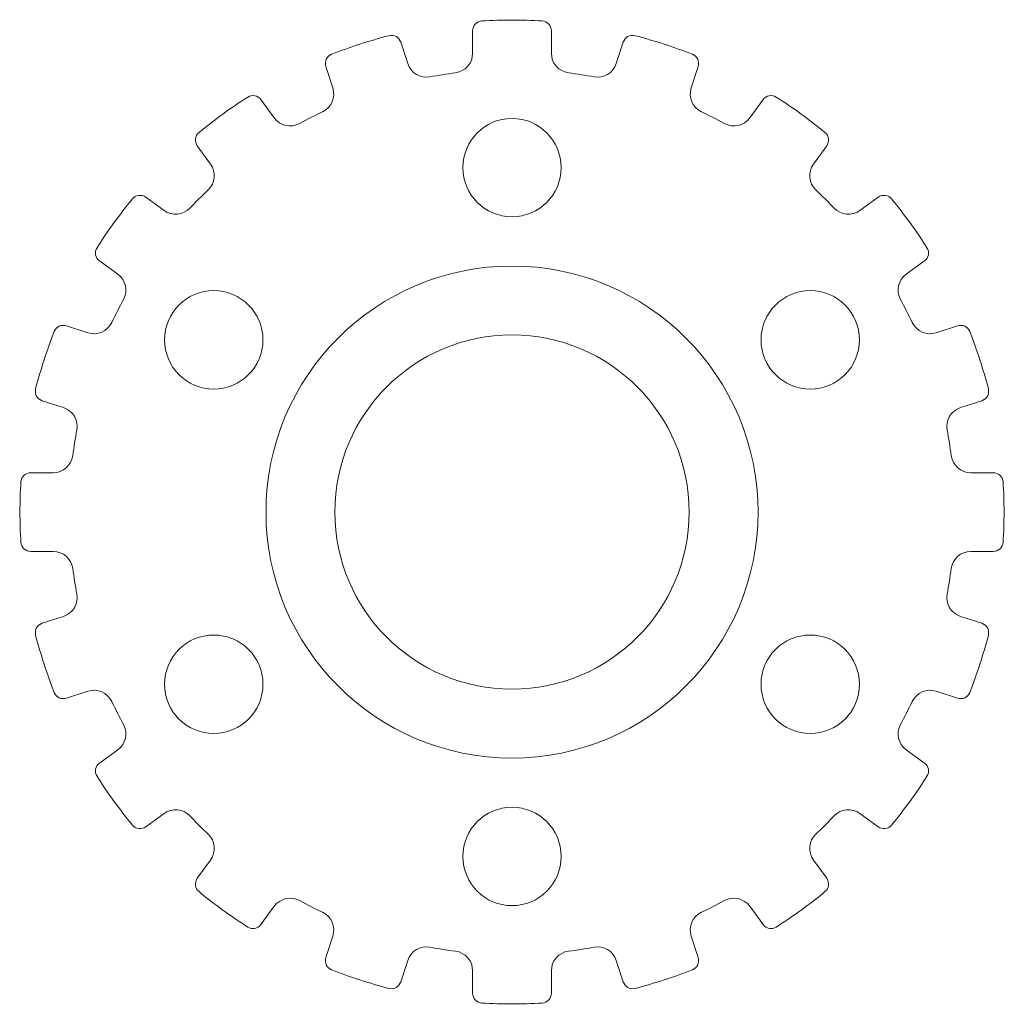
# Model space of a CAD drawing. Units: millimetres. Extents: x 3111 to 3211, y 1416 to 1516.
import ezdxf

# ---------------------------------------------------------------- set-up
doc = ezdxf.new("R2010")
doc.units = ezdxf.units.MM
doc.layers.add('M-CONS', color=8, linetype='Continuous', lineweight=18)

# ---------------------------------------------------------------- blocks, each defined once
blk = doc.blocks.new('*U1')
blk.add_lwpolyline([(-5.74, -2.68, 0.377199), (-4, -0.7), (-4, 1.59, -0.396382), (-3.06, 2.59, -0.030641), (3.06, 2.59, -0.396382), (4, 1.59), (4, -0.7, 0.377199), (5.74, -2.68)], format="xyb")
blk = doc.blocks.new('*U2')
at = {"layer": 'M-CONS', "color": 0, "linetype": 'ByBlock', "lineweight": -2, "transparency": 16777216}
for p, rotation in [((3146.51, 1510.65), 17.99999999999998), ((3175.75, 1510.65), 342), ((3133.32, 1503.93), 36.00000000000001), ((3188.94, 1503.93), 324), ((3122.85, 1493.47), 54), ((3199.41, 1493.47), 306), ((3116.13, 1480.28), 72), ((3206.13, 1480.28), 288), ((3113.81, 1465.65), 90), ((3208.45, 1465.65), 270), ((3116.13, 1451.03), 108), ((3206.13, 1451.03), 252), ((3122.85, 1437.84), 126), ((3199.41, 1437.84), 234), ((3133.32, 1427.37), 144), ((3188.94, 1427.37), 216), ((3146.51, 1420.65), 162), ((3175.75, 1420.65), 198), ((3161.13, 1418.34), 180)]:
    blk.add_blockref('*U1', p, dxfattribs=dict(at, rotation=rotation))
blk.add_blockref('*U1', (3161.13, 1512.97), dxfattribs=at)
blk = doc.blocks.new('*U3')
blk.add_circle((0, 0), 5)
blk = doc.blocks.new('*U4')
at = {"layer": 'M-CONS', "color": 0, "linetype": 'ByBlock', "lineweight": -2, "transparency": 16777216}
blk.add_blockref('*U3', (3161.13, 1500.65), dxfattribs=at)
for p, rotation in [((3130.82, 1483.15), 59.99999999999999), ((3191.44, 1483.15), 300), ((3130.82, 1448.15), 120), ((3191.44, 1448.15), 240), ((3161.13, 1430.65), 180)]:
    blk.add_blockref('*U3', p, dxfattribs=dict(at, rotation=rotation))

msp = doc.modelspace()

# ---------------------------------------------------------------- linework, layer by layer
at = {"layer": 'M-CONS'}
for radius in [25, 18]:
    msp.add_circle((3161.13, 1465.65), radius, dxfattribs=at)
for start, end in [(97.3344, 100.6656), (79.3344, 82.6656), (115.3344, 118.6656), (61.3344, 64.6656), (133.3344, 136.6656), (43.3344, 46.6656), (151.3344, 154.6656), (25.3344, 28.6656), (169.3344, 172.6656), (7.3344, 10.6656), (187.3344, 190.6656), (349.3344, 352.6656), (205.3344, 208.6656), (331.3344, 334.6656), (223.3344, 226.6656), (313.3344, 316.6656), (241.3344, 244.6656), (295.3344, 298.6656), (259.3344, 262.6656), (277.3344, 280.6656)]:
    msp.add_arc((3161.13, 1465.65), 45, start, end, dxfattribs=at)

# ---------------------------------------------------------------- block references
for name in ['*U2', '*U4']:
    msp.add_blockref(name, (0, 0), dxfattribs=at)

doc.saveas('drawing.dxf')
